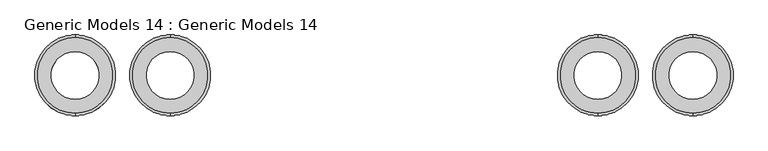
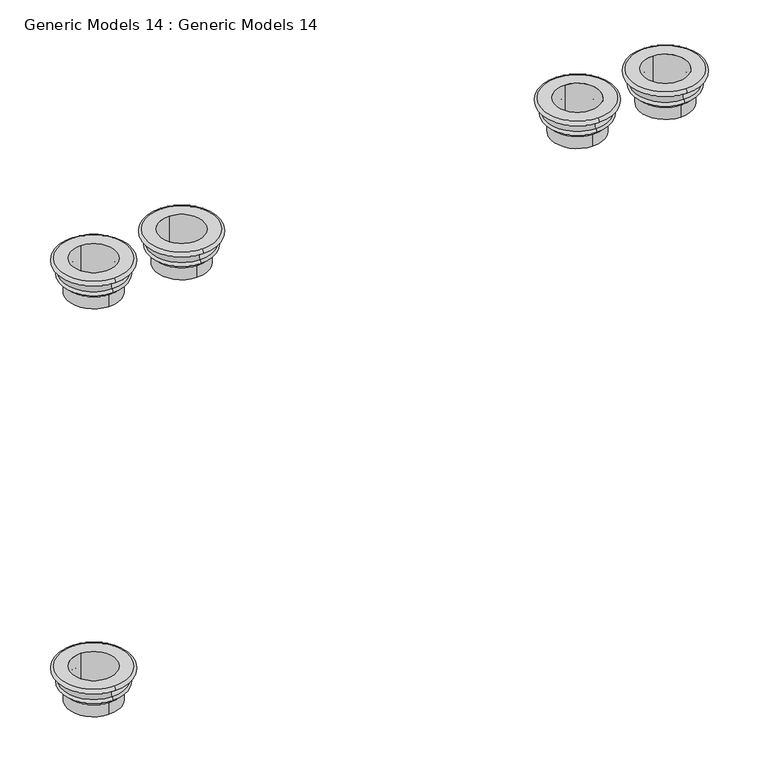
"""IFC4 building model written with IfcOpenShell, lengths in millimetres: proxy geometry, Generic Models 14 : Generic Models 14."""

from ifc_helpers import new_model, si_unit, point, frame, origin, place, context, project, spatial, polyline, circle_curve, ellipse_curve, trimmed, source, transform, mapped, element, save
from ifc_brep_helpers import plane_surface, cylinder_surface, revolved_surface, advanced_brep


def generic_models_14_generic_models_14_9f9ef7df(model_context):
    return source(origin(), model_context, "Body", "AdvancedBrep", [
        advanced_brep(
        [(-2563.6825076, -7335.7292912, 4826.0), (-2563.6825076, -7742.1292912, 4826.0), (-2563.6825076, -7742.1292912, 4851.4), (-2563.6825076, -7335.7292912, 4851.4), (-2563.6825076, -7356.4126296, 4774.291654), (-2563.6825076, -7721.4459527, 4774.291654), (-2563.6825076, -7361.1292912, 4749.8), (-2563.6825076, -7716.7292912, 4749.8), (-2563.6825076, -7386.5292912, 4724.4), (-2563.6825076, -7691.3292912, 4724.4), (-2563.6825076, -7691.3292912, 4749.8), (-2563.6825076, -7386.5292912, 4749.8), (-2563.6825076, -7386.5292912, 4648.2), (-2563.6825076, -7691.3292912, 4648.2), (-2563.6825076, -7411.9292912, 4851.4), (-2563.6825076, -7665.9292912, 4851.4), (-2563.6825076, -7665.9292912, 4648.2), (-2563.6825076, -7411.9292912, 4648.2)],
        [
            (0, 1, circle_curve(frame((-2563.6825076, -7538.9292912, 4826.0), z_axis=(0.0, 0.0, 1.0), x_axis=(0.0, -1.0, 0.0)), 203.2)),
            (1, 2, circle_curve(frame((-2563.6825076, -7742.1292912, 4838.7), z_axis=(-1.0, 0.0, 0.0), x_axis=(0.0, -1.0, 0.0)), 12.7)),
            (2, 3, circle_curve(frame((-2563.6825076, -7538.9292912, 4851.4), z_axis=(0.0, 0.0, -1.0), x_axis=(0.0, -1.0, 0.0)), 203.2)),
            (3, 0, circle_curve(frame((-2563.6825076, -7335.7292912, 4838.7), z_axis=(-1.0, 0.0, 0.0), x_axis=(0.0, 1.0, 0.0)), 12.7)),
            (4, 5, circle_curve(frame((-2563.6825076, -7538.9292912, 4774.291654), z_axis=(0.0, 0.0, 1.0), x_axis=(0.0, -1.0, 0.0)), 182.5166616)),
            (5, 1, circle_curve(frame((-2563.6825076, -7742.1292912, 4796.0091593), z_axis=(1.0, 0.0, 0.0), x_axis=(0.0, -1.0, 0.0)), 29.9908407)),
            (0, 4, circle_curve(frame((-2563.6825076, -7335.7292912, 4796.0091593), z_axis=(1.0, 0.0, 0.0), x_axis=(0.0, 1.0, 0.0)), 29.9908407)),
            (6, 7, circle_curve(frame((-2563.6825076, -7538.9292912, 4749.8), z_axis=(0.0, 0.0, 1.0), x_axis=(0.0, -1.0, 0.0)), 177.8)),
            (7, 5, circle_curve(frame((-2563.6825076, -7716.7292912, 4762.5), z_axis=(-1.0, 0.0, 0.0), x_axis=(0.0, -1.0, 0.0)), 12.7)),
            (4, 6, circle_curve(frame((-2563.6825076, -7361.1292912, 4762.5), z_axis=(-1.0, 0.0, 0.0), x_axis=(0.0, 1.0, 0.0)), 12.7)),
            (8, 9, circle_curve(frame((-2563.6825076, -7538.9292912, 4724.4), z_axis=(0.0, 0.0, 1.0), x_axis=(0.0, -1.0, 0.0)), 152.4)),
            (9, 10, circle_curve(frame((-2563.6825076, -7691.3292912, 4737.1), z_axis=(-1.0, 0.0, 0.0), x_axis=(0.0, -1.0, 0.0)), 12.7)),
            (10, 11, circle_curve(frame((-2563.6825076, -7538.9292912, 4749.8), z_axis=(0.0, 0.0, -1.0), x_axis=(0.0, -1.0, 0.0)), 152.4)),
            (11, 8, circle_curve(frame((-2563.6825076, -7386.5292912, 4737.1), z_axis=(-1.0, 0.0, 0.0), x_axis=(0.0, 1.0, 0.0)), 12.7)),
            (12, 13, circle_curve(frame((-2563.6825076, -7538.9292912, 4648.2), z_axis=(0.0, 0.0, 1.0), x_axis=(0.0, -1.0, 0.0)), 152.4)),
            (13, 9),
            (8, 12),
            (14, 15, circle_curve(frame((-2563.6825076, -7538.9292912, 4851.4), z_axis=(0.0, 0.0, 1.0), x_axis=(0.0, -1.0, 0.0)), 127.0)),
            (15, 16),
            (16, 17, circle_curve(frame((-2563.6825076, -7538.9292912, 4648.2), z_axis=(0.0, 0.0, -1.0), x_axis=(0.0, -1.0, 0.0)), 127.0)),
            (17, 14),
            (1, 0, circle_curve(frame((-2563.6825076, -7538.9292912, 4826.0), z_axis=(0.0, 0.0, 1.0), x_axis=(0.0, 1.0, 0.0)), 203.2)),
            (3, 2, circle_curve(frame((-2563.6825076, -7538.9292912, 4851.4), z_axis=(0.0, 0.0, -1.0), x_axis=(0.0, 1.0, 0.0)), 203.2)),
            (5, 4, circle_curve(frame((-2563.6825076, -7538.9292912, 4774.291654), z_axis=(0.0, 0.0, 1.0), x_axis=(0.0, 1.0, 0.0)), 182.5166616)),
            (7, 6, circle_curve(frame((-2563.6825076, -7538.9292912, 4749.8), z_axis=(0.0, 0.0, 1.0), x_axis=(0.0, 1.0, 0.0)), 177.8)),
            (10, 11, circle_curve(frame((-2563.6825076, -7538.9292912, 4749.8), z_axis=(0.0, 0.0, 1.0), x_axis=(0.0, 1.0, 0.0)), 152.4)),
            (9, 8, circle_curve(frame((-2563.6825076, -7538.9292912, 4724.4), z_axis=(0.0, 0.0, 1.0), x_axis=(0.0, 1.0, 0.0)), 152.4)),
            (13, 12, circle_curve(frame((-2563.6825076, -7538.9292912, 4648.2), z_axis=(0.0, 0.0, 1.0), x_axis=(0.0, 1.0, 0.0)), 152.4)),
            (16, 17, circle_curve(frame((-2563.6825076, -7538.9292912, 4648.2), z_axis=(0.0, 0.0, 1.0), x_axis=(0.0, 1.0, 0.0)), 127.0)),
            (15, 14, circle_curve(frame((-2563.6825076, -7538.9292912, 4851.4), z_axis=(0.0, 0.0, 1.0), x_axis=(0.0, 1.0, 0.0)), 127.0)),
        ],
        [
            revolved_surface(trimmed(ellipse_curve(frame((-2563.6825076, -7742.1292912, 4838.7), z_axis=(1.0, 0.0, 0.0), x_axis=(0.0, -1.0, 0.0)), 12.7, 12.7), [point((-2563.6825076, -7742.1292912, 4851.4))], [point((-2563.6825076, -7742.1292912, 4826.0))], True, "CARTESIAN"), (-2563.6825076, -7538.9292912, 4851.4), (0.0, 0.0, -1.0)),
            revolved_surface(trimmed(ellipse_curve(frame((-2563.6825076, -7742.1292912, 4796.0091593), z_axis=(-1.0, 0.0, 0.0), x_axis=(0.0, -1.0, 0.0)), 29.9908407, 29.9908407), [point((-2563.6825076, -7742.1292912, 4826.0))], [point((-2563.6825076, -7721.4459527, 4774.291654))], True, "CARTESIAN"), (-2563.6825076, -7538.9292912, 4851.4), (0.0, 0.0, -1.0)),
            revolved_surface(trimmed(ellipse_curve(frame((-2563.6825076, -7716.7292912, 4762.5), z_axis=(1.0, 0.0, 0.0), x_axis=(0.0, -1.0, 0.0)), 12.7, 12.7), [point((-2563.6825076, -7721.4459527, 4774.291654))], [point((-2563.6825076, -7716.7292912, 4749.8))], True, "CARTESIAN"), (-2563.6825076, -7538.9292912, 4851.4), (0.0, 0.0, -1.0)),
            revolved_surface(trimmed(ellipse_curve(frame((-2563.6825076, -7691.3292912, 4737.1), z_axis=(1.0, 0.0, 0.0), x_axis=(0.0, -1.0, 0.0)), 12.7, 12.7), [point((-2563.6825076, -7691.3292912, 4749.8))], [point((-2563.6825076, -7691.3292912, 4724.4))], True, "CARTESIAN"), (-2563.6825076, -7538.9292912, 4851.4), (0.0, 0.0, -1.0)),
            cylinder_surface(frame((-2563.6825076, -7538.9292912, 4851.4), z_axis=(0.0, 0.0, -1.0), x_axis=(0.0, -1.0, 0.0)), 152.4),
            revolved_surface(polyline([(-2563.6825076, -7665.9292912, 4648.2), (-2563.6825076, -7665.9292912, 4851.4)]), (-2563.6825076, -7538.9292912, 4851.4), (0.0, 0.0, -1.0)),
            revolved_surface(trimmed(ellipse_curve(frame((-2563.6825076, -7335.7292912, 4838.7), z_axis=(-1.0, 0.0, 0.0), x_axis=(0.0, 1.0, 0.0)), 12.7, 12.7), [point((-2563.6825076, -7335.7292912, 4851.4))], [point((-2563.6825076, -7335.7292912, 4826.0))], True, "CARTESIAN"), (-2563.6825076, -7538.9292912, 4851.4), (0.0, 0.0, -1.0)),
            revolved_surface(trimmed(ellipse_curve(frame((-2563.6825076, -7335.7292912, 4796.0091593), z_axis=(1.0, 0.0, 0.0), x_axis=(0.0, 1.0, 0.0)), 29.9908407, 29.9908407), [point((-2563.6825076, -7335.7292912, 4826.0))], [point((-2563.6825076, -7356.4126296, 4774.291654))], True, "CARTESIAN"), (-2563.6825076, -7538.9292912, 4851.4), (0.0, 0.0, -1.0)),
            revolved_surface(trimmed(ellipse_curve(frame((-2563.6825076, -7361.1292912, 4762.5), z_axis=(-1.0, 0.0, 0.0), x_axis=(0.0, 1.0, 0.0)), 12.7, 12.7), [point((-2563.6825076, -7356.4126296, 4774.291654))], [point((-2563.6825076, -7361.1292912, 4749.8))], True, "CARTESIAN"), (-2563.6825076, -7538.9292912, 4851.4), (0.0, 0.0, -1.0)),
            plane_surface(frame((-2563.6825076, -7538.9292912, 4749.8), z_axis=(0.0, 0.0, -1.0), x_axis=(0.0, 1.0, 0.0))),
            revolved_surface(trimmed(ellipse_curve(frame((-2563.6825076, -7386.5292912, 4737.1), z_axis=(-1.0, 0.0, 0.0), x_axis=(0.0, 1.0, 0.0)), 12.7, 12.7), [point((-2563.6825076, -7386.5292912, 4749.8))], [point((-2563.6825076, -7386.5292912, 4724.4))], True, "CARTESIAN"), (-2563.6825076, -7538.9292912, 4851.4), (0.0, 0.0, -1.0)),
            cylinder_surface(frame((-2563.6825076, -7538.9292912, 4851.4), z_axis=(0.0, 0.0, -1.0), x_axis=(0.0, 1.0, 0.0)), 152.4),
            plane_surface(frame((-2563.6825076, -7538.9292912, 4648.2), z_axis=(0.0, 0.0, -1.0), x_axis=(0.0, 1.0, 0.0))),
            revolved_surface(polyline([(-2563.6825076, -7411.9292912, 4648.2), (-2563.6825076, -7411.9292912, 4851.4)]), (-2563.6825076, -7538.9292912, 4851.4), (0.0, 0.0, -1.0)),
            plane_surface(frame((-2563.6825076, -7538.9292912, 4851.4), z_axis=(0.0, 0.0, 1.0), x_axis=(0.0, 1.0, 0.0))),
        ],
        [
            (0, [[1, 2, 3, 4]]),
            (1, [[5, 6, -1, 7]]),
            (2, [[8, 9, -5, 10]]),
            (3, [[11, 12, 13, 14]]),
            (4, [[15, 16, -11, 17]]),
            (5, [[18, 19, 20, 21]]),
            (6, [[22, -4, 23, -2]]),
            (7, [[24, -7, -22, -6]]),
            (8, [[25, -10, -24, -9]]),
            (9, [[-25, -8], [26, -13]]),
            (10, [[27, -14, -26, -12]]),
            (11, [[28, -17, -27, -16]]),
            (12, [[-28, -15], [29, -20]]),
            (13, [[30, -21, -29, -19]]),
            (14, [[-23, -3], [-30, -18]]),
        ],
    ),
        advanced_brep(
        [(-2055.6825076, -7335.7292912, 4826.0), (-2055.6825076, -7742.1292912, 4826.0), (-2055.6825076, -7742.1292912, 4851.4), (-2055.6825076, -7335.7292912, 4851.4), (-2055.6825076, -7356.4126296, 4774.291654), (-2055.6825076, -7721.4459527, 4774.291654), (-2055.6825076, -7361.1292912, 4749.8), (-2055.6825076, -7716.7292912, 4749.8), (-2055.6825076, -7386.5292912, 4724.4), (-2055.6825076, -7691.3292912, 4724.4), (-2055.6825076, -7691.3292912, 4749.8), (-2055.6825076, -7386.5292912, 4749.8), (-2055.6825076, -7386.5292912, 4648.2), (-2055.6825076, -7691.3292912, 4648.2), (-2055.6825076, -7411.9292912, 4851.4), (-2055.6825076, -7665.9292912, 4851.4), (-2055.6825076, -7665.9292912, 4648.2), (-2055.6825076, -7411.9292912, 4648.2)],
        [
            (0, 1, circle_curve(frame((-2055.6825076, -7538.9292912, 4826.0), z_axis=(0.0, 0.0, 1.0), x_axis=(0.0, -1.0, 0.0)), 203.2)),
            (1, 2, circle_curve(frame((-2055.6825076, -7742.1292912, 4838.7), z_axis=(-1.0, 0.0, 0.0), x_axis=(0.0, -1.0, 0.0)), 12.7)),
            (2, 3, circle_curve(frame((-2055.6825076, -7538.9292912, 4851.4), z_axis=(0.0, 0.0, -1.0), x_axis=(0.0, -1.0, 0.0)), 203.2)),
            (3, 0, circle_curve(frame((-2055.6825076, -7335.7292912, 4838.7), z_axis=(-1.0, 0.0, 0.0), x_axis=(0.0, 1.0, 0.0)), 12.7)),
            (4, 5, circle_curve(frame((-2055.6825076, -7538.9292912, 4774.291654), z_axis=(0.0, 0.0, 1.0), x_axis=(0.0, -1.0, 0.0)), 182.5166616)),
            (5, 1, circle_curve(frame((-2055.6825076, -7742.1292912, 4796.0091593), z_axis=(1.0, 0.0, 0.0), x_axis=(0.0, -1.0, 0.0)), 29.9908407)),
            (0, 4, circle_curve(frame((-2055.6825076, -7335.7292912, 4796.0091593), z_axis=(1.0, 0.0, 0.0), x_axis=(0.0, 1.0, 0.0)), 29.9908407)),
            (6, 7, circle_curve(frame((-2055.6825076, -7538.9292912, 4749.8), z_axis=(0.0, 0.0, 1.0), x_axis=(0.0, -1.0, 0.0)), 177.8)),
            (7, 5, circle_curve(frame((-2055.6825076, -7716.7292912, 4762.5), z_axis=(-1.0, 0.0, 0.0), x_axis=(0.0, -1.0, 0.0)), 12.7)),
            (4, 6, circle_curve(frame((-2055.6825076, -7361.1292912, 4762.5), z_axis=(-1.0, 0.0, 0.0), x_axis=(0.0, 1.0, 0.0)), 12.7)),
            (8, 9, circle_curve(frame((-2055.6825076, -7538.9292912, 4724.4), z_axis=(0.0, 0.0, 1.0), x_axis=(0.0, -1.0, 0.0)), 152.4)),
            (9, 10, circle_curve(frame((-2055.6825076, -7691.3292912, 4737.1), z_axis=(-1.0, 0.0, 0.0), x_axis=(0.0, -1.0, 0.0)), 12.7)),
            (10, 11, circle_curve(frame((-2055.6825076, -7538.9292912, 4749.8), z_axis=(0.0, 0.0, -1.0), x_axis=(0.0, -1.0, 0.0)), 152.4)),
            (11, 8, circle_curve(frame((-2055.6825076, -7386.5292912, 4737.1), z_axis=(-1.0, 0.0, 0.0), x_axis=(0.0, 1.0, 0.0)), 12.7)),
            (12, 13, circle_curve(frame((-2055.6825076, -7538.9292912, 4648.2), z_axis=(0.0, 0.0, 1.0), x_axis=(0.0, -1.0, 0.0)), 152.4)),
            (13, 9),
            (8, 12),
            (14, 15, circle_curve(frame((-2055.6825076, -7538.9292912, 4851.4), z_axis=(0.0, 0.0, 1.0), x_axis=(0.0, -1.0, 0.0)), 127.0)),
            (15, 16),
            (16, 17, circle_curve(frame((-2055.6825076, -7538.9292912, 4648.2), z_axis=(0.0, 0.0, -1.0), x_axis=(0.0, -1.0, 0.0)), 127.0)),
            (17, 14),
            (1, 0, circle_curve(frame((-2055.6825076, -7538.9292912, 4826.0), z_axis=(0.0, 0.0, 1.0), x_axis=(0.0, 1.0, 0.0)), 203.2)),
            (3, 2, circle_curve(frame((-2055.6825076, -7538.9292912, 4851.4), z_axis=(0.0, 0.0, -1.0), x_axis=(0.0, 1.0, 0.0)), 203.2)),
            (5, 4, circle_curve(frame((-2055.6825076, -7538.9292912, 4774.291654), z_axis=(0.0, 0.0, 1.0), x_axis=(0.0, 1.0, 0.0)), 182.5166616)),
            (7, 6, circle_curve(frame((-2055.6825076, -7538.9292912, 4749.8), z_axis=(0.0, 0.0, 1.0), x_axis=(0.0, 1.0, 0.0)), 177.8)),
            (10, 11, circle_curve(frame((-2055.6825076, -7538.9292912, 4749.8), z_axis=(0.0, 0.0, 1.0), x_axis=(0.0, 1.0, 0.0)), 152.4)),
            (9, 8, circle_curve(frame((-2055.6825076, -7538.9292912, 4724.4), z_axis=(0.0, 0.0, 1.0), x_axis=(0.0, 1.0, 0.0)), 152.4)),
            (13, 12, circle_curve(frame((-2055.6825076, -7538.9292912, 4648.2), z_axis=(0.0, 0.0, 1.0), x_axis=(0.0, 1.0, 0.0)), 152.4)),
            (16, 17, circle_curve(frame((-2055.6825076, -7538.9292912, 4648.2), z_axis=(0.0, 0.0, 1.0), x_axis=(0.0, 1.0, 0.0)), 127.0)),
            (15, 14, circle_curve(frame((-2055.6825076, -7538.9292912, 4851.4), z_axis=(0.0, 0.0, 1.0), x_axis=(0.0, 1.0, 0.0)), 127.0)),
        ],
        [
            revolved_surface(trimmed(ellipse_curve(frame((-2055.6825076, -7742.1292912, 4838.7), z_axis=(1.0, 0.0, 0.0), x_axis=(0.0, -1.0, 0.0)), 12.7, 12.7), [point((-2055.6825076, -7742.1292912, 4851.4))], [point((-2055.6825076, -7742.1292912, 4826.0))], True, "CARTESIAN"), (-2055.6825076, -7538.9292912, 4851.4), (0.0, 0.0, -1.0)),
            revolved_surface(trimmed(ellipse_curve(frame((-2055.6825076, -7742.1292912, 4796.0091593), z_axis=(-1.0, 0.0, 0.0), x_axis=(0.0, -1.0, 0.0)), 29.9908407, 29.9908407), [point((-2055.6825076, -7742.1292912, 4826.0))], [point((-2055.6825076, -7721.4459527, 4774.291654))], True, "CARTESIAN"), (-2055.6825076, -7538.9292912, 4851.4), (0.0, 0.0, -1.0)),
            revolved_surface(trimmed(ellipse_curve(frame((-2055.6825076, -7716.7292912, 4762.5), z_axis=(1.0, 0.0, 0.0), x_axis=(0.0, -1.0, 0.0)), 12.7, 12.7), [point((-2055.6825076, -7721.4459527, 4774.291654))], [point((-2055.6825076, -7716.7292912, 4749.8))], True, "CARTESIAN"), (-2055.6825076, -7538.9292912, 4851.4), (0.0, 0.0, -1.0)),
            revolved_surface(trimmed(ellipse_curve(frame((-2055.6825076, -7691.3292912, 4737.1), z_axis=(1.0, 0.0, 0.0), x_axis=(0.0, -1.0, 0.0)), 12.7, 12.7), [point((-2055.6825076, -7691.3292912, 4749.8))], [point((-2055.6825076, -7691.3292912, 4724.4))], True, "CARTESIAN"), (-2055.6825076, -7538.9292912, 4851.4), (0.0, 0.0, -1.0)),
            cylinder_surface(frame((-2055.6825076, -7538.9292912, 4851.4), z_axis=(0.0, 0.0, -1.0), x_axis=(0.0, -1.0, 0.0)), 152.4),
            revolved_surface(polyline([(-2055.6825076, -7665.9292912, 4648.2), (-2055.6825076, -7665.9292912, 4851.4)]), (-2055.6825076, -7538.9292912, 4851.4), (0.0, 0.0, -1.0)),
            revolved_surface(trimmed(ellipse_curve(frame((-2055.6825076, -7335.7292912, 4838.7), z_axis=(-1.0, 0.0, 0.0), x_axis=(0.0, 1.0, 0.0)), 12.7, 12.7), [point((-2055.6825076, -7335.7292912, 4851.4))], [point((-2055.6825076, -7335.7292912, 4826.0))], True, "CARTESIAN"), (-2055.6825076, -7538.9292912, 4851.4), (0.0, 0.0, -1.0)),
            revolved_surface(trimmed(ellipse_curve(frame((-2055.6825076, -7335.7292912, 4796.0091593), z_axis=(1.0, 0.0, 0.0), x_axis=(0.0, 1.0, 0.0)), 29.9908407, 29.9908407), [point((-2055.6825076, -7335.7292912, 4826.0))], [point((-2055.6825076, -7356.4126296, 4774.291654))], True, "CARTESIAN"), (-2055.6825076, -7538.9292912, 4851.4), (0.0, 0.0, -1.0)),
            revolved_surface(trimmed(ellipse_curve(frame((-2055.6825076, -7361.1292912, 4762.5), z_axis=(-1.0, 0.0, 0.0), x_axis=(0.0, 1.0, 0.0)), 12.7, 12.7), [point((-2055.6825076, -7356.4126296, 4774.291654))], [point((-2055.6825076, -7361.1292912, 4749.8))], True, "CARTESIAN"), (-2055.6825076, -7538.9292912, 4851.4), (0.0, 0.0, -1.0)),
            plane_surface(frame((-2055.6825076, -7538.9292912, 4749.8), z_axis=(0.0, 0.0, -1.0), x_axis=(0.0, 1.0, 0.0))),
            revolved_surface(trimmed(ellipse_curve(frame((-2055.6825076, -7386.5292912, 4737.1), z_axis=(-1.0, 0.0, 0.0), x_axis=(0.0, 1.0, 0.0)), 12.7, 12.7), [point((-2055.6825076, -7386.5292912, 4749.8))], [point((-2055.6825076, -7386.5292912, 4724.4))], True, "CARTESIAN"), (-2055.6825076, -7538.9292912, 4851.4), (0.0, 0.0, -1.0)),
            cylinder_surface(frame((-2055.6825076, -7538.9292912, 4851.4), z_axis=(0.0, 0.0, -1.0), x_axis=(0.0, 1.0, 0.0)), 152.4),
            plane_surface(frame((-2055.6825076, -7538.9292912, 4648.2), z_axis=(0.0, 0.0, -1.0), x_axis=(0.0, 1.0, 0.0))),
            revolved_surface(polyline([(-2055.6825076, -7411.9292912, 4648.2), (-2055.6825076, -7411.9292912, 4851.4)]), (-2055.6825076, -7538.9292912, 4851.4), (0.0, 0.0, -1.0)),
            plane_surface(frame((-2055.6825076, -7538.9292912, 4851.4), z_axis=(0.0, 0.0, 1.0), x_axis=(0.0, 1.0, 0.0))),
        ],
        [
            (0, [[1, 2, 3, 4]]),
            (1, [[5, 6, -1, 7]]),
            (2, [[8, 9, -5, 10]]),
            (3, [[11, 12, 13, 14]]),
            (4, [[15, 16, -11, 17]]),
            (5, [[18, 19, 20, 21]]),
            (6, [[22, -4, 23, -2]]),
            (7, [[24, -7, -22, -6]]),
            (8, [[25, -10, -24, -9]]),
            (9, [[-25, -8], [26, -13]]),
            (10, [[27, -14, -26, -12]]),
            (11, [[28, -17, -27, -16]]),
            (12, [[-28, -15], [29, -20]]),
            (13, [[30, -21, -29, -19]]),
            (14, [[-23, -3], [-30, -18]]),
        ],
    ),
        advanced_brep(
        [(230.3174924, -7335.7292912, 4826.0), (230.3174924, -7742.1292912, 4826.0), (230.3174924, -7742.1292912, 4851.4), (230.3174924, -7335.7292912, 4851.4), (230.3174924, -7356.4126296, 4774.291654), (230.3174924, -7721.4459527, 4774.291654), (230.3174924, -7361.1292912, 4749.8), (230.3174924, -7716.7292912, 4749.8), (230.3174924, -7386.5292912, 4724.4), (230.3174924, -7691.3292912, 4724.4), (230.3174924, -7691.3292912, 4749.8), (230.3174924, -7386.5292912, 4749.8), (230.3174924, -7386.5292912, 4648.2), (230.3174924, -7691.3292912, 4648.2), (230.3174924, -7411.9292912, 4851.4), (230.3174924, -7665.9292912, 4851.4), (230.3174924, -7665.9292912, 4648.2), (230.3174924, -7411.9292912, 4648.2)],
        [
            (0, 1, circle_curve(frame((230.3174924, -7538.9292912, 4826.0), z_axis=(0.0, 0.0, 1.0), x_axis=(0.0, -1.0, 0.0)), 203.2)),
            (1, 2, circle_curve(frame((230.3174924, -7742.1292912, 4838.7), z_axis=(-1.0, 0.0, 0.0), x_axis=(0.0, -1.0, 0.0)), 12.7)),
            (2, 3, circle_curve(frame((230.3174924, -7538.9292912, 4851.4), z_axis=(0.0, 0.0, -1.0), x_axis=(0.0, -1.0, 0.0)), 203.2)),
            (3, 0, circle_curve(frame((230.3174924, -7335.7292912, 4838.7), z_axis=(-1.0, 0.0, 0.0), x_axis=(0.0, 1.0, 0.0)), 12.7)),
            (4, 5, circle_curve(frame((230.3174924, -7538.9292912, 4774.291654), z_axis=(0.0, 0.0, 1.0), x_axis=(0.0, -1.0, 0.0)), 182.5166616)),
            (5, 1, circle_curve(frame((230.3174924, -7742.1292912, 4796.0091593), z_axis=(1.0, 0.0, 0.0), x_axis=(0.0, -1.0, 0.0)), 29.9908407)),
            (0, 4, circle_curve(frame((230.3174924, -7335.7292912, 4796.0091593), z_axis=(1.0, 0.0, 0.0), x_axis=(0.0, 1.0, 0.0)), 29.9908407)),
            (6, 7, circle_curve(frame((230.3174924, -7538.9292912, 4749.8), z_axis=(0.0, 0.0, 1.0), x_axis=(0.0, -1.0, 0.0)), 177.8)),
            (7, 5, circle_curve(frame((230.3174924, -7716.7292912, 4762.5), z_axis=(-1.0, 0.0, 0.0), x_axis=(0.0, -1.0, 0.0)), 12.7)),
            (4, 6, circle_curve(frame((230.3174924, -7361.1292912, 4762.5), z_axis=(-1.0, 0.0, 0.0), x_axis=(0.0, 1.0, 0.0)), 12.7)),
            (8, 9, circle_curve(frame((230.3174924, -7538.9292912, 4724.4), z_axis=(0.0, 0.0, 1.0), x_axis=(0.0, -1.0, 0.0)), 152.4)),
            (9, 10, circle_curve(frame((230.3174924, -7691.3292912, 4737.1), z_axis=(-1.0, 0.0, 0.0), x_axis=(0.0, -1.0, 0.0)), 12.7)),
            (10, 11, circle_curve(frame((230.3174924, -7538.9292912, 4749.8), z_axis=(0.0, 0.0, -1.0), x_axis=(0.0, -1.0, 0.0)), 152.4)),
            (11, 8, circle_curve(frame((230.3174924, -7386.5292912, 4737.1), z_axis=(-1.0, 0.0, 0.0), x_axis=(0.0, 1.0, 0.0)), 12.7)),
            (12, 13, circle_curve(frame((230.3174924, -7538.9292912, 4648.2), z_axis=(0.0, 0.0, 1.0), x_axis=(0.0, -1.0, 0.0)), 152.4)),
            (13, 9),
            (8, 12),
            (14, 15, circle_curve(frame((230.3174924, -7538.9292912, 4851.4), z_axis=(0.0, 0.0, 1.0), x_axis=(0.0, -1.0, 0.0)), 127.0)),
            (15, 16),
            (16, 17, circle_curve(frame((230.3174924, -7538.9292912, 4648.2), z_axis=(0.0, 0.0, -1.0), x_axis=(0.0, -1.0, 0.0)), 127.0)),
            (17, 14),
            (1, 0, circle_curve(frame((230.3174924, -7538.9292912, 4826.0), z_axis=(0.0, 0.0, 1.0), x_axis=(0.0, 1.0, 0.0)), 203.2)),
            (3, 2, circle_curve(frame((230.3174924, -7538.9292912, 4851.4), z_axis=(0.0, 0.0, -1.0), x_axis=(0.0, 1.0, 0.0)), 203.2)),
            (5, 4, circle_curve(frame((230.3174924, -7538.9292912, 4774.291654), z_axis=(0.0, 0.0, 1.0), x_axis=(0.0, 1.0, 0.0)), 182.5166616)),
            (7, 6, circle_curve(frame((230.3174924, -7538.9292912, 4749.8), z_axis=(0.0, 0.0, 1.0), x_axis=(0.0, 1.0, 0.0)), 177.8)),
            (10, 11, circle_curve(frame((230.3174924, -7538.9292912, 4749.8), z_axis=(0.0, 0.0, 1.0), x_axis=(0.0, 1.0, 0.0)), 152.4)),
            (9, 8, circle_curve(frame((230.3174924, -7538.9292912, 4724.4), z_axis=(0.0, 0.0, 1.0), x_axis=(0.0, 1.0, 0.0)), 152.4)),
            (13, 12, circle_curve(frame((230.3174924, -7538.9292912, 4648.2), z_axis=(0.0, 0.0, 1.0), x_axis=(0.0, 1.0, 0.0)), 152.4)),
            (16, 17, circle_curve(frame((230.3174924, -7538.9292912, 4648.2), z_axis=(0.0, 0.0, 1.0), x_axis=(0.0, 1.0, 0.0)), 127.0)),
            (15, 14, circle_curve(frame((230.3174924, -7538.9292912, 4851.4), z_axis=(0.0, 0.0, 1.0), x_axis=(0.0, 1.0, 0.0)), 127.0)),
        ],
        [
            revolved_surface(trimmed(ellipse_curve(frame((230.3174924, -7742.1292912, 4838.7), z_axis=(1.0, 0.0, 0.0), x_axis=(0.0, -1.0, 0.0)), 12.7, 12.7), [point((230.3174924, -7742.1292912, 4851.4))], [point((230.3174924, -7742.1292912, 4826.0))], True, "CARTESIAN"), (230.3174924, -7538.9292912, 4851.4), (0.0, 0.0, -1.0)),
            revolved_surface(trimmed(ellipse_curve(frame((230.3174924, -7742.1292912, 4796.0091593), z_axis=(-1.0, 0.0, 0.0), x_axis=(0.0, -1.0, 0.0)), 29.9908407, 29.9908407), [point((230.3174924, -7742.1292912, 4826.0))], [point((230.3174924, -7721.4459527, 4774.291654))], True, "CARTESIAN"), (230.3174924, -7538.9292912, 4851.4), (0.0, 0.0, -1.0)),
            revolved_surface(trimmed(ellipse_curve(frame((230.3174924, -7716.7292912, 4762.5), z_axis=(1.0, 0.0, 0.0), x_axis=(0.0, -1.0, 0.0)), 12.7, 12.7), [point((230.3174924, -7721.4459527, 4774.291654))], [point((230.3174924, -7716.7292912, 4749.8))], True, "CARTESIAN"), (230.3174924, -7538.9292912, 4851.4), (0.0, 0.0, -1.0)),
            revolved_surface(trimmed(ellipse_curve(frame((230.3174924, -7691.3292912, 4737.1), z_axis=(1.0, 0.0, 0.0), x_axis=(0.0, -1.0, 0.0)), 12.7, 12.7), [point((230.3174924, -7691.3292912, 4749.8))], [point((230.3174924, -7691.3292912, 4724.4))], True, "CARTESIAN"), (230.3174924, -7538.9292912, 4851.4), (0.0, 0.0, -1.0)),
            cylinder_surface(frame((230.3174924, -7538.9292912, 4851.4), z_axis=(0.0, 0.0, -1.0), x_axis=(0.0, -1.0, 0.0)), 152.4),
            revolved_surface(polyline([(230.3174924, -7665.9292912, 4648.2), (230.3174924, -7665.9292912, 4851.4)]), (230.3174924, -7538.9292912, 4851.4), (0.0, 0.0, -1.0)),
            revolved_surface(trimmed(ellipse_curve(frame((230.3174924, -7335.7292912, 4838.7), z_axis=(-1.0, 0.0, 0.0), x_axis=(0.0, 1.0, 0.0)), 12.7, 12.7), [point((230.3174924, -7335.7292912, 4851.4))], [point((230.3174924, -7335.7292912, 4826.0))], True, "CARTESIAN"), (230.3174924, -7538.9292912, 4851.4), (0.0, 0.0, -1.0)),
            revolved_surface(trimmed(ellipse_curve(frame((230.3174924, -7335.7292912, 4796.0091593), z_axis=(1.0, 0.0, 0.0), x_axis=(0.0, 1.0, 0.0)), 29.9908407, 29.9908407), [point((230.3174924, -7335.7292912, 4826.0))], [point((230.3174924, -7356.4126296, 4774.291654))], True, "CARTESIAN"), (230.3174924, -7538.9292912, 4851.4), (0.0, 0.0, -1.0)),
            revolved_surface(trimmed(ellipse_curve(frame((230.3174924, -7361.1292912, 4762.5), z_axis=(-1.0, 0.0, 0.0), x_axis=(0.0, 1.0, 0.0)), 12.7, 12.7), [point((230.3174924, -7356.4126296, 4774.291654))], [point((230.3174924, -7361.1292912, 4749.8))], True, "CARTESIAN"), (230.3174924, -7538.9292912, 4851.4), (0.0, 0.0, -1.0)),
            plane_surface(frame((230.3174924, -7538.9292912, 4749.8), z_axis=(0.0, 0.0, -1.0), x_axis=(0.0, 1.0, 0.0))),
            revolved_surface(trimmed(ellipse_curve(frame((230.3174924, -7386.5292912, 4737.1), z_axis=(-1.0, 0.0, 0.0), x_axis=(0.0, 1.0, 0.0)), 12.7, 12.7), [point((230.3174924, -7386.5292912, 4749.8))], [point((230.3174924, -7386.5292912, 4724.4))], True, "CARTESIAN"), (230.3174924, -7538.9292912, 4851.4), (0.0, 0.0, -1.0)),
            cylinder_surface(frame((230.3174924, -7538.9292912, 4851.4), z_axis=(0.0, 0.0, -1.0), x_axis=(0.0, 1.0, 0.0)), 152.4),
            plane_surface(frame((230.3174924, -7538.9292912, 4648.2), z_axis=(0.0, 0.0, -1.0), x_axis=(0.0, 1.0, 0.0))),
            revolved_surface(polyline([(230.3174924, -7411.9292912, 4648.2), (230.3174924, -7411.9292912, 4851.4)]), (230.3174924, -7538.9292912, 4851.4), (0.0, 0.0, -1.0)),
            plane_surface(frame((230.3174924, -7538.9292912, 4851.4), z_axis=(0.0, 0.0, 1.0), x_axis=(0.0, 1.0, 0.0))),
        ],
        [
            (0, [[1, 2, 3, 4]]),
            (1, [[5, 6, -1, 7]]),
            (2, [[8, 9, -5, 10]]),
            (3, [[11, 12, 13, 14]]),
            (4, [[15, 16, -11, 17]]),
            (5, [[18, 19, 20, 21]]),
            (6, [[22, -4, 23, -2]]),
            (7, [[24, -7, -22, -6]]),
            (8, [[25, -10, -24, -9]]),
            (9, [[-25, -8], [26, -13]]),
            (10, [[27, -14, -26, -12]]),
            (11, [[28, -17, -27, -16]]),
            (12, [[-28, -15], [29, -20]]),
            (13, [[30, -21, -29, -19]]),
            (14, [[-23, -3], [-30, -18]]),
        ],
    ),
        advanced_brep(
        [(738.3174924, -7335.7292912, 4826.0), (738.3174924, -7742.1292912, 4826.0), (738.3174924, -7742.1292912, 4851.4), (738.3174924, -7335.7292912, 4851.4), (738.3174924, -7356.4126296, 4774.291654), (738.3174924, -7721.4459527, 4774.291654), (738.3174924, -7361.1292912, 4749.8), (738.3174924, -7716.7292912, 4749.8), (738.3174924, -7386.5292912, 4724.4), (738.3174924, -7691.3292912, 4724.4), (738.3174924, -7691.3292912, 4749.8), (738.3174924, -7386.5292912, 4749.8), (738.3174924, -7386.5292912, 4648.2), (738.3174924, -7691.3292912, 4648.2), (738.3174924, -7411.9292912, 4851.4), (738.3174924, -7665.9292912, 4851.4), (738.3174924, -7665.9292912, 4648.2), (738.3174924, -7411.9292912, 4648.2)],
        [
            (0, 1, circle_curve(frame((738.3174924, -7538.9292912, 4826.0), z_axis=(0.0, 0.0, 1.0), x_axis=(0.0, -1.0, 0.0)), 203.2)),
            (1, 2, circle_curve(frame((738.3174924, -7742.1292912, 4838.7), z_axis=(-1.0, 0.0, 0.0), x_axis=(0.0, -1.0, 0.0)), 12.7)),
            (2, 3, circle_curve(frame((738.3174924, -7538.9292912, 4851.4), z_axis=(0.0, 0.0, -1.0), x_axis=(0.0, -1.0, 0.0)), 203.2)),
            (3, 0, circle_curve(frame((738.3174924, -7335.7292912, 4838.7), z_axis=(-1.0, 0.0, 0.0), x_axis=(0.0, 1.0, 0.0)), 12.7)),
            (4, 5, circle_curve(frame((738.3174924, -7538.9292912, 4774.291654), z_axis=(0.0, 0.0, 1.0), x_axis=(0.0, -1.0, 0.0)), 182.5166616)),
            (5, 1, circle_curve(frame((738.3174924, -7742.1292912, 4796.0091593), z_axis=(1.0, 0.0, 0.0), x_axis=(0.0, -1.0, 0.0)), 29.9908407)),
            (0, 4, circle_curve(frame((738.3174924, -7335.7292912, 4796.0091593), z_axis=(1.0, 0.0, 0.0), x_axis=(0.0, 1.0, 0.0)), 29.9908407)),
            (6, 7, circle_curve(frame((738.3174924, -7538.9292912, 4749.8), z_axis=(0.0, 0.0, 1.0), x_axis=(0.0, -1.0, 0.0)), 177.8)),
            (7, 5, circle_curve(frame((738.3174924, -7716.7292912, 4762.5), z_axis=(-1.0, 0.0, 0.0), x_axis=(0.0, -1.0, 0.0)), 12.7)),
            (4, 6, circle_curve(frame((738.3174924, -7361.1292912, 4762.5), z_axis=(-1.0, 0.0, 0.0), x_axis=(0.0, 1.0, 0.0)), 12.7)),
            (8, 9, circle_curve(frame((738.3174924, -7538.9292912, 4724.4), z_axis=(0.0, 0.0, 1.0), x_axis=(0.0, -1.0, 0.0)), 152.4)),
            (9, 10, circle_curve(frame((738.3174924, -7691.3292912, 4737.1), z_axis=(-1.0, 0.0, 0.0), x_axis=(0.0, -1.0, 0.0)), 12.7)),
            (10, 11, circle_curve(frame((738.3174924, -7538.9292912, 4749.8), z_axis=(0.0, 0.0, -1.0), x_axis=(0.0, -1.0, 0.0)), 152.4)),
            (11, 8, circle_curve(frame((738.3174924, -7386.5292912, 4737.1), z_axis=(-1.0, 0.0, 0.0), x_axis=(0.0, 1.0, 0.0)), 12.7)),
            (12, 13, circle_curve(frame((738.3174924, -7538.9292912, 4648.2), z_axis=(0.0, 0.0, 1.0), x_axis=(0.0, -1.0, 0.0)), 152.4)),
            (13, 9),
            (8, 12),
            (14, 15, circle_curve(frame((738.3174924, -7538.9292912, 4851.4), z_axis=(0.0, 0.0, 1.0), x_axis=(0.0, -1.0, 0.0)), 127.0)),
            (15, 16),
            (16, 17, circle_curve(frame((738.3174924, -7538.9292912, 4648.2), z_axis=(0.0, 0.0, -1.0), x_axis=(0.0, -1.0, 0.0)), 127.0)),
            (17, 14),
            (1, 0, circle_curve(frame((738.3174924, -7538.9292912, 4826.0), z_axis=(0.0, 0.0, 1.0), x_axis=(0.0, 1.0, 0.0)), 203.2)),
            (3, 2, circle_curve(frame((738.3174924, -7538.9292912, 4851.4), z_axis=(0.0, 0.0, -1.0), x_axis=(0.0, 1.0, 0.0)), 203.2)),
            (5, 4, circle_curve(frame((738.3174924, -7538.9292912, 4774.291654), z_axis=(0.0, 0.0, 1.0), x_axis=(0.0, 1.0, 0.0)), 182.5166616)),
            (7, 6, circle_curve(frame((738.3174924, -7538.9292912, 4749.8), z_axis=(0.0, 0.0, 1.0), x_axis=(0.0, 1.0, 0.0)), 177.8)),
            (10, 11, circle_curve(frame((738.3174924, -7538.9292912, 4749.8), z_axis=(0.0, 0.0, 1.0), x_axis=(0.0, 1.0, 0.0)), 152.4)),
            (9, 8, circle_curve(frame((738.3174924, -7538.9292912, 4724.4), z_axis=(0.0, 0.0, 1.0), x_axis=(0.0, 1.0, 0.0)), 152.4)),
            (13, 12, circle_curve(frame((738.3174924, -7538.9292912, 4648.2), z_axis=(0.0, 0.0, 1.0), x_axis=(0.0, 1.0, 0.0)), 152.4)),
            (16, 17, circle_curve(frame((738.3174924, -7538.9292912, 4648.2), z_axis=(0.0, 0.0, 1.0), x_axis=(0.0, 1.0, 0.0)), 127.0)),
            (15, 14, circle_curve(frame((738.3174924, -7538.9292912, 4851.4), z_axis=(0.0, 0.0, 1.0), x_axis=(0.0, 1.0, 0.0)), 127.0)),
        ],
        [
            revolved_surface(trimmed(ellipse_curve(frame((738.3174924, -7742.1292912, 4838.7), z_axis=(1.0, 0.0, 0.0), x_axis=(0.0, -1.0, 0.0)), 12.7, 12.7), [point((738.3174924, -7742.1292912, 4851.4))], [point((738.3174924, -7742.1292912, 4826.0))], True, "CARTESIAN"), (738.3174924, -7538.9292912, 4851.4), (0.0, 0.0, -1.0)),
            revolved_surface(trimmed(ellipse_curve(frame((738.3174924, -7742.1292912, 4796.0091593), z_axis=(-1.0, 0.0, 0.0), x_axis=(0.0, -1.0, 0.0)), 29.9908407, 29.9908407), [point((738.3174924, -7742.1292912, 4826.0))], [point((738.3174924, -7721.4459527, 4774.291654))], True, "CARTESIAN"), (738.3174924, -7538.9292912, 4851.4), (0.0, 0.0, -1.0)),
            revolved_surface(trimmed(ellipse_curve(frame((738.3174924, -7716.7292912, 4762.5), z_axis=(1.0, 0.0, 0.0), x_axis=(0.0, -1.0, 0.0)), 12.7, 12.7), [point((738.3174924, -7721.4459527, 4774.291654))], [point((738.3174924, -7716.7292912, 4749.8))], True, "CARTESIAN"), (738.3174924, -7538.9292912, 4851.4), (0.0, 0.0, -1.0)),
            revolved_surface(trimmed(ellipse_curve(frame((738.3174924, -7691.3292912, 4737.1), z_axis=(1.0, 0.0, 0.0), x_axis=(0.0, -1.0, 0.0)), 12.7, 12.7), [point((738.3174924, -7691.3292912, 4749.8))], [point((738.3174924, -7691.3292912, 4724.4))], True, "CARTESIAN"), (738.3174924, -7538.9292912, 4851.4), (0.0, 0.0, -1.0)),
            cylinder_surface(frame((738.3174924, -7538.9292912, 4851.4), z_axis=(0.0, 0.0, -1.0), x_axis=(0.0, -1.0, 0.0)), 152.4),
            revolved_surface(polyline([(738.3174924, -7665.9292912, 4648.2), (738.3174924, -7665.9292912, 4851.4)]), (738.3174924, -7538.9292912, 4851.4), (0.0, 0.0, -1.0)),
            revolved_surface(trimmed(ellipse_curve(frame((738.3174924, -7335.7292912, 4838.7), z_axis=(-1.0, 0.0, 0.0), x_axis=(0.0, 1.0, 0.0)), 12.7, 12.7), [point((738.3174924, -7335.7292912, 4851.4))], [point((738.3174924, -7335.7292912, 4826.0))], True, "CARTESIAN"), (738.3174924, -7538.9292912, 4851.4), (0.0, 0.0, -1.0)),
            revolved_surface(trimmed(ellipse_curve(frame((738.3174924, -7335.7292912, 4796.0091593), z_axis=(1.0, 0.0, 0.0), x_axis=(0.0, 1.0, 0.0)), 29.9908407, 29.9908407), [point((738.3174924, -7335.7292912, 4826.0))], [point((738.3174924, -7356.4126296, 4774.291654))], True, "CARTESIAN"), (738.3174924, -7538.9292912, 4851.4), (0.0, 0.0, -1.0)),
            revolved_surface(trimmed(ellipse_curve(frame((738.3174924, -7361.1292912, 4762.5), z_axis=(-1.0, 0.0, 0.0), x_axis=(0.0, 1.0, 0.0)), 12.7, 12.7), [point((738.3174924, -7356.4126296, 4774.291654))], [point((738.3174924, -7361.1292912, 4749.8))], True, "CARTESIAN"), (738.3174924, -7538.9292912, 4851.4), (0.0, 0.0, -1.0)),
            plane_surface(frame((738.3174924, -7538.9292912, 4749.8), z_axis=(0.0, 0.0, -1.0), x_axis=(0.0, 1.0, 0.0))),
            revolved_surface(trimmed(ellipse_curve(frame((738.3174924, -7386.5292912, 4737.1), z_axis=(-1.0, 0.0, 0.0), x_axis=(0.0, 1.0, 0.0)), 12.7, 12.7), [point((738.3174924, -7386.5292912, 4749.8))], [point((738.3174924, -7386.5292912, 4724.4))], True, "CARTESIAN"), (738.3174924, -7538.9292912, 4851.4), (0.0, 0.0, -1.0)),
            cylinder_surface(frame((738.3174924, -7538.9292912, 4851.4), z_axis=(0.0, 0.0, -1.0), x_axis=(0.0, 1.0, 0.0)), 152.4),
            plane_surface(frame((738.3174924, -7538.9292912, 4648.2), z_axis=(0.0, 0.0, -1.0), x_axis=(0.0, 1.0, 0.0))),
            revolved_surface(polyline([(738.3174924, -7411.9292912, 4648.2), (738.3174924, -7411.9292912, 4851.4)]), (738.3174924, -7538.9292912, 4851.4), (0.0, 0.0, -1.0)),
            plane_surface(frame((738.3174924, -7538.9292912, 4851.4), z_axis=(0.0, 0.0, 1.0), x_axis=(0.0, 1.0, 0.0))),
        ],
        [
            (0, [[1, 2, 3, 4]]),
            (1, [[5, 6, -1, 7]]),
            (2, [[8, 9, -5, 10]]),
            (3, [[11, 12, 13, 14]]),
            (4, [[15, 16, -11, 17]]),
            (5, [[18, 19, 20, 21]]),
            (6, [[22, -4, 23, -2]]),
            (7, [[24, -7, -22, -6]]),
            (8, [[25, -10, -24, -9]]),
            (9, [[-25, -8], [26, -13]]),
            (10, [[27, -14, -26, -12]]),
            (11, [[28, -17, -27, -16]]),
            (12, [[-28, -15], [29, -20]]),
            (13, [[30, -21, -29, -19]]),
            (14, [[-23, -3], [-30, -18]]),
        ],
    ),
        advanced_brep(
        [(-2563.6825076, -7335.7292912, 2336.8), (-2563.6825076, -7742.1292912, 2336.8), (-2563.6825076, -7742.1292912, 2362.2), (-2563.6825076, -7335.7292912, 2362.2), (-2563.6825076, -7356.4126296, 2285.091654), (-2563.6825076, -7721.4459527, 2285.091654), (-2563.6825076, -7361.1292912, 2260.6), (-2563.6825076, -7716.7292912, 2260.6), (-2563.6825076, -7386.5292912, 2235.2), (-2563.6825076, -7691.3292912, 2235.2), (-2563.6825076, -7691.3292912, 2260.6), (-2563.6825076, -7386.5292912, 2260.6), (-2563.6825076, -7386.5292912, 2159.0), (-2563.6825076, -7691.3292912, 2159.0), (-2563.6825076, -7411.9292912, 2362.2), (-2563.6825076, -7665.9292912, 2362.2), (-2563.6825076, -7665.9292912, 2159.0), (-2563.6825076, -7411.9292912, 2159.0)],
        [
            (0, 1, circle_curve(frame((-2563.6825076, -7538.9292912, 2336.8), z_axis=(0.0, 0.0, 1.0), x_axis=(0.0, -1.0, 0.0)), 203.2)),
            (1, 2, circle_curve(frame((-2563.6825076, -7742.1292912, 2349.5), z_axis=(-1.0, 0.0, 0.0), x_axis=(0.0, -1.0, 0.0)), 12.7)),
            (2, 3, circle_curve(frame((-2563.6825076, -7538.9292912, 2362.2), z_axis=(0.0, 0.0, -1.0), x_axis=(0.0, -1.0, 0.0)), 203.2)),
            (3, 0, circle_curve(frame((-2563.6825076, -7335.7292912, 2349.5), z_axis=(-1.0, 0.0, 0.0), x_axis=(0.0, 1.0, 0.0)), 12.7)),
            (4, 5, circle_curve(frame((-2563.6825076, -7538.9292912, 2285.091654), z_axis=(0.0, 0.0, 1.0), x_axis=(0.0, -1.0, 0.0)), 182.5166616)),
            (5, 1, circle_curve(frame((-2563.6825076, -7742.1292912, 2306.8091593), z_axis=(1.0, 0.0, 0.0), x_axis=(0.0, -1.0, 0.0)), 29.9908407)),
            (0, 4, circle_curve(frame((-2563.6825076, -7335.7292912, 2306.8091593), z_axis=(1.0, 0.0, 0.0), x_axis=(0.0, 1.0, 0.0)), 29.9908407)),
            (6, 7, circle_curve(frame((-2563.6825076, -7538.9292912, 2260.6), z_axis=(0.0, 0.0, 1.0), x_axis=(0.0, -1.0, 0.0)), 177.8)),
            (7, 5, circle_curve(frame((-2563.6825076, -7716.7292912, 2273.3), z_axis=(-1.0, 0.0, 0.0), x_axis=(0.0, -1.0, 0.0)), 12.7)),
            (4, 6, circle_curve(frame((-2563.6825076, -7361.1292912, 2273.3), z_axis=(-1.0, 0.0, 0.0), x_axis=(0.0, 1.0, 0.0)), 12.7)),
            (8, 9, circle_curve(frame((-2563.6825076, -7538.9292912, 2235.2), z_axis=(0.0, 0.0, 1.0), x_axis=(0.0, -1.0, 0.0)), 152.4)),
            (9, 10, circle_curve(frame((-2563.6825076, -7691.3292912, 2247.9), z_axis=(-1.0, 0.0, 0.0), x_axis=(0.0, -1.0, 0.0)), 12.7)),
            (10, 11, circle_curve(frame((-2563.6825076, -7538.9292912, 2260.6), z_axis=(0.0, 0.0, -1.0), x_axis=(0.0, -1.0, 0.0)), 152.4)),
            (11, 8, circle_curve(frame((-2563.6825076, -7386.5292912, 2247.9), z_axis=(-1.0, 0.0, 0.0), x_axis=(0.0, 1.0, 0.0)), 12.7)),
            (12, 13, circle_curve(frame((-2563.6825076, -7538.9292912, 2159.0), z_axis=(0.0, 0.0, 1.0), x_axis=(0.0, -1.0, 0.0)), 152.4)),
            (13, 9),
            (8, 12),
            (14, 15, circle_curve(frame((-2563.6825076, -7538.9292912, 2362.2), z_axis=(0.0, 0.0, 1.0), x_axis=(0.0, -1.0, 0.0)), 127.0)),
            (15, 16),
            (16, 17, circle_curve(frame((-2563.6825076, -7538.9292912, 2159.0), z_axis=(0.0, 0.0, -1.0), x_axis=(0.0, -1.0, 0.0)), 127.0)),
            (17, 14),
            (1, 0, circle_curve(frame((-2563.6825076, -7538.9292912, 2336.8), z_axis=(0.0, 0.0, 1.0), x_axis=(0.0, 1.0, 0.0)), 203.2)),
            (3, 2, circle_curve(frame((-2563.6825076, -7538.9292912, 2362.2), z_axis=(0.0, 0.0, -1.0), x_axis=(0.0, 1.0, 0.0)), 203.2)),
            (5, 4, circle_curve(frame((-2563.6825076, -7538.9292912, 2285.091654), z_axis=(0.0, 0.0, 1.0), x_axis=(0.0, 1.0, 0.0)), 182.5166616)),
            (7, 6, circle_curve(frame((-2563.6825076, -7538.9292912, 2260.6), z_axis=(0.0, 0.0, 1.0), x_axis=(0.0, 1.0, 0.0)), 177.8)),
            (10, 11, circle_curve(frame((-2563.6825076, -7538.9292912, 2260.6), z_axis=(0.0, 0.0, 1.0), x_axis=(0.0, 1.0, 0.0)), 152.4)),
            (9, 8, circle_curve(frame((-2563.6825076, -7538.9292912, 2235.2), z_axis=(0.0, 0.0, 1.0), x_axis=(0.0, 1.0, 0.0)), 152.4)),
            (13, 12, circle_curve(frame((-2563.6825076, -7538.9292912, 2159.0), z_axis=(0.0, 0.0, 1.0), x_axis=(0.0, 1.0, 0.0)), 152.4)),
            (16, 17, circle_curve(frame((-2563.6825076, -7538.9292912, 2159.0), z_axis=(0.0, 0.0, 1.0), x_axis=(0.0, 1.0, 0.0)), 127.0)),
            (15, 14, circle_curve(frame((-2563.6825076, -7538.9292912, 2362.2), z_axis=(0.0, 0.0, 1.0), x_axis=(0.0, 1.0, 0.0)), 127.0)),
        ],
        [
            revolved_surface(trimmed(ellipse_curve(frame((-2563.6825076, -7742.1292912, 2349.5), z_axis=(1.0, 0.0, 0.0), x_axis=(0.0, -1.0, 0.0)), 12.7, 12.7), [point((-2563.6825076, -7742.1292912, 2362.2))], [point((-2563.6825076, -7742.1292912, 2336.8))], True, "CARTESIAN"), (-2563.6825076, -7538.9292912, 2362.2), (0.0, 0.0, -1.0)),
            revolved_surface(trimmed(ellipse_curve(frame((-2563.6825076, -7742.1292912, 2306.8091593), z_axis=(-1.0, 0.0, 0.0), x_axis=(0.0, -1.0, 0.0)), 29.9908407, 29.9908407), [point((-2563.6825076, -7742.1292912, 2336.8))], [point((-2563.6825076, -7721.4459527, 2285.091654))], True, "CARTESIAN"), (-2563.6825076, -7538.9292912, 2362.2), (0.0, 0.0, -1.0)),
            revolved_surface(trimmed(ellipse_curve(frame((-2563.6825076, -7716.7292912, 2273.3), z_axis=(1.0, 0.0, 0.0), x_axis=(0.0, -1.0, 0.0)), 12.7, 12.7), [point((-2563.6825076, -7721.4459527, 2285.091654))], [point((-2563.6825076, -7716.7292912, 2260.6))], True, "CARTESIAN"), (-2563.6825076, -7538.9292912, 2362.2), (0.0, 0.0, -1.0)),
            revolved_surface(trimmed(ellipse_curve(frame((-2563.6825076, -7691.3292912, 2247.9), z_axis=(1.0, 0.0, 0.0), x_axis=(0.0, -1.0, 0.0)), 12.7, 12.7), [point((-2563.6825076, -7691.3292912, 2260.6))], [point((-2563.6825076, -7691.3292912, 2235.2))], True, "CARTESIAN"), (-2563.6825076, -7538.9292912, 2362.2), (0.0, 0.0, -1.0)),
            cylinder_surface(frame((-2563.6825076, -7538.9292912, 2362.2), z_axis=(0.0, 0.0, -1.0), x_axis=(0.0, -1.0, 0.0)), 152.4),
            revolved_surface(polyline([(-2563.6825076, -7665.9292912, 2159.0), (-2563.6825076, -7665.9292912, 2362.2)]), (-2563.6825076, -7538.9292912, 2362.2), (0.0, 0.0, -1.0)),
            revolved_surface(trimmed(ellipse_curve(frame((-2563.6825076, -7335.7292912, 2349.5), z_axis=(-1.0, 0.0, 0.0), x_axis=(0.0, 1.0, 0.0)), 12.7, 12.7), [point((-2563.6825076, -7335.7292912, 2362.2))], [point((-2563.6825076, -7335.7292912, 2336.8))], True, "CARTESIAN"), (-2563.6825076, -7538.9292912, 2362.2), (0.0, 0.0, -1.0)),
            revolved_surface(trimmed(ellipse_curve(frame((-2563.6825076, -7335.7292912, 2306.8091593), z_axis=(1.0, 0.0, 0.0), x_axis=(0.0, 1.0, 0.0)), 29.9908407, 29.9908407), [point((-2563.6825076, -7335.7292912, 2336.8))], [point((-2563.6825076, -7356.4126296, 2285.091654))], True, "CARTESIAN"), (-2563.6825076, -7538.9292912, 2362.2), (0.0, 0.0, -1.0)),
            revolved_surface(trimmed(ellipse_curve(frame((-2563.6825076, -7361.1292912, 2273.3), z_axis=(-1.0, 0.0, 0.0), x_axis=(0.0, 1.0, 0.0)), 12.7, 12.7), [point((-2563.6825076, -7356.4126296, 2285.091654))], [point((-2563.6825076, -7361.1292912, 2260.6))], True, "CARTESIAN"), (-2563.6825076, -7538.9292912, 2362.2), (0.0, 0.0, -1.0)),
            plane_surface(frame((-2563.6825076, -7538.9292912, 2260.6), z_axis=(0.0, 0.0, -1.0), x_axis=(0.0, 1.0, 0.0))),
            revolved_surface(trimmed(ellipse_curve(frame((-2563.6825076, -7386.5292912, 2247.9), z_axis=(-1.0, 0.0, 0.0), x_axis=(0.0, 1.0, 0.0)), 12.7, 12.7), [point((-2563.6825076, -7386.5292912, 2260.6))], [point((-2563.6825076, -7386.5292912, 2235.2))], True, "CARTESIAN"), (-2563.6825076, -7538.9292912, 2362.2), (0.0, 0.0, -1.0)),
            cylinder_surface(frame((-2563.6825076, -7538.9292912, 2362.2), z_axis=(0.0, 0.0, -1.0), x_axis=(0.0, 1.0, 0.0)), 152.4),
            plane_surface(frame((-2563.6825076, -7538.9292912, 2159.0), z_axis=(0.0, 0.0, -1.0), x_axis=(0.0, 1.0, 0.0))),
            revolved_surface(polyline([(-2563.6825076, -7411.9292912, 2159.0), (-2563.6825076, -7411.9292912, 2362.2)]), (-2563.6825076, -7538.9292912, 2362.2), (0.0, 0.0, -1.0)),
            plane_surface(frame((-2563.6825076, -7538.9292912, 2362.2), z_axis=(0.0, 0.0, 1.0), x_axis=(0.0, 1.0, 0.0))),
        ],
        [
            (0, [[1, 2, 3, 4]]),
            (1, [[5, 6, -1, 7]]),
            (2, [[8, 9, -5, 10]]),
            (3, [[11, 12, 13, 14]]),
            (4, [[15, 16, -11, 17]]),
            (5, [[18, 19, 20, 21]]),
            (6, [[22, -4, 23, -2]]),
            (7, [[24, -7, -22, -6]]),
            (8, [[25, -10, -24, -9]]),
            (9, [[-25, -8], [26, -13]]),
            (10, [[27, -14, -26, -12]]),
            (11, [[28, -17, -27, -16]]),
            (12, [[-28, -15], [29, -20]]),
            (13, [[30, -21, -29, -19]]),
            (14, [[-23, -3], [-30, -18]]),
        ],
    ),
    ])


if __name__ == "__main__":
    model = new_model("IFC4")
    model_context = context("Model", 3, world=origin())
    ifc_project = project(units=[si_unit("LENGTHUNIT", "METRE", prefix="MILLI")], contexts=[model_context])
    site = spatial("IfcSite", under=ifc_project)
    building = spatial("IfcBuilding", under=site)
    placement = place(None, origin())
    generic_models_14_generic_models_14_shape = generic_models_14_generic_models_14_9f9ef7df(model_context)
    element("IfcBuildingElementProxy", 1, Name="Generic Models 14 : Generic Models 14", ObjectType="Generic Models 14 : Generic Models 14", at=placement, inside=building, context=model_context, shape_type="MappedRepresentation", body=[
        mapped(generic_models_14_generic_models_14_shape, transform((0.0, 0.0, 0.0), x_axis=(1.0, 0.0, 0.0), y_axis=(0.0, 1.0, 0.0), z_axis=(0.0, 0.0, 1.0))),
    ])
    save(model, "model.ifc")
